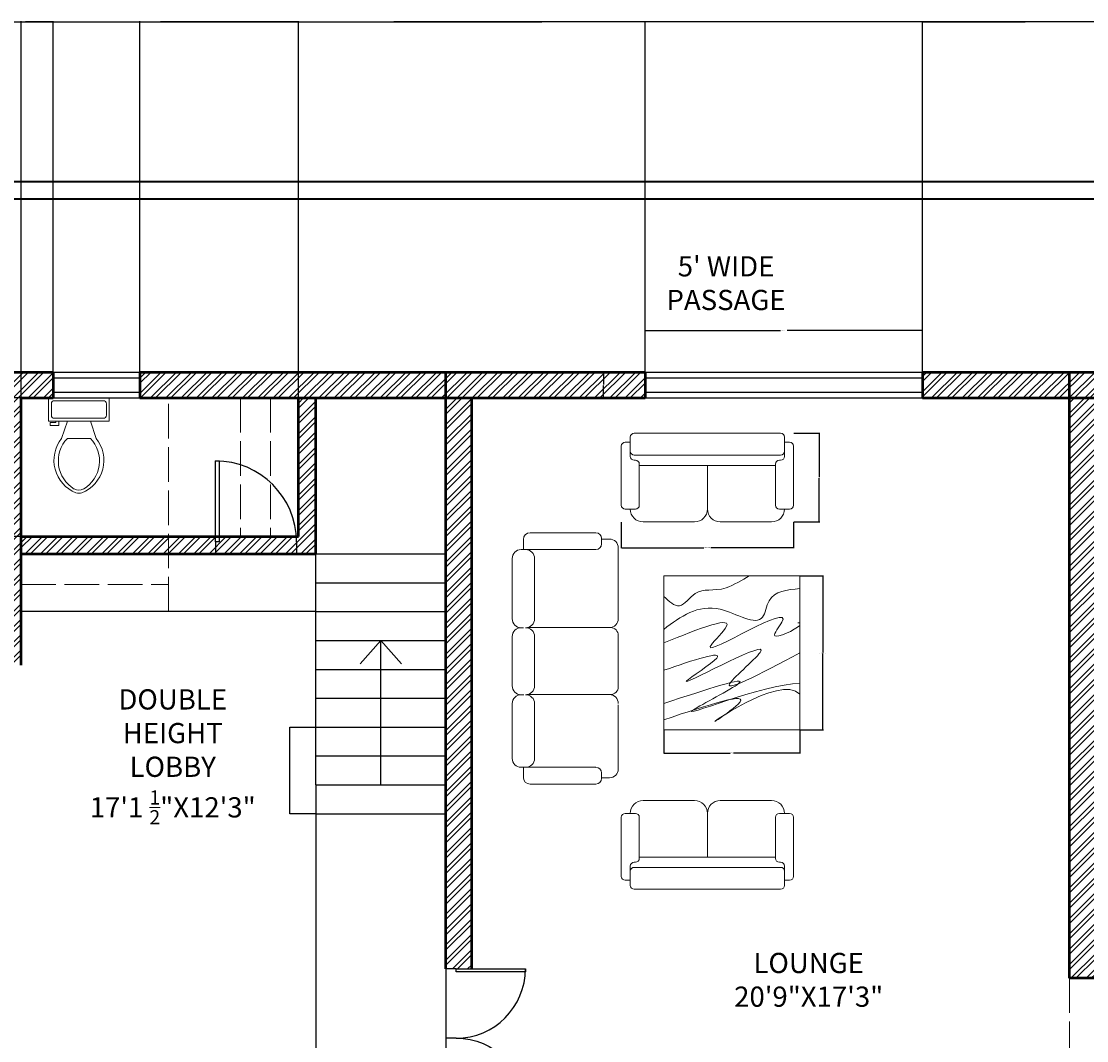
# Model space of a CAD drawing. Units: inches. Extents: x -249 to 953, y -127 to 590.
# Tile 3 of 4: x 171 to 540, y 237 to 590. Entities that reach past the tile are written whole.
import ezdxf

# ---------------------------------------------------------------- set-up
doc = ezdxf.new("R2010")
doc.units = ezdxf.units.IN
doc.header["$MEASUREMENT"] = 0
doc.linetypes.add('ACAD_ISO02W100', pattern=[15, 12, -3])
for name, color, linetype, lineweight in [('A-ANNO-DIMS', 2, 'Continuous', 18), ('A-AREA-IDEN', 2, 'Continuous', 18), ('A-FLOR-STRS', 4, 'Continuous', 25), ('A-FLOR-STRS-OVHD', 4, 'ACAD_ISO02W100', 18), ('A-FURN', 42, 'Continuous', 18), ('A-GLAZ', 5, 'Continuous', 25), ('A-WALL', 7, 'Continuous', 50), ('A-WALL-OVHD', 7, 'ACAD_ISO02W100', 18), ('A-WALL-PATT', 8, 'Continuous', 13), ('C-PROP', 7, 'Continuous', 35), ('DOOR', 22, 'Continuous', 25), ('L-ANNO-TEXT', 2, 'Continuous', 18), ('WASHROOM', 2, 'Continuous', 18)]:
    doc.layers.add(name, color=color, linetype=linetype, lineweight=lineweight)
doc.styles.get("Standard").update_dxf_attribs({"font": 'arial.ttf'})
doc.dimstyles.get("Standard").update_dxf_attribs({"dimtxt": 0.18, "dimasz": 0.18, "dimexe": 0.18, "dimexo": 0.0625, "dimgap": 0.09, "dimtad": 0, "dimtih": 1, "dimtoh": 1, "dimdec": 4, "dimzin": 0, "dimdsep": 46, "dimtxsty": 'Standard', "dimcen": 0.09, "dimadec": 0, "dimazin": 0, "dimtfac": 1, "dimtdec": 4, "dimtofl": 0, "dimtmove": 0, "dimatfit": 3, "dimfxl": 1, "dimtolj": 1, "dimtzin": 0, "dimarcsym": 0})

# ---------------------------------------------------------------- blocks, each defined once
blk = doc.blocks.new('*U2')
for p, q in [((0, 0), (0, -6)), ((40, 0), (40, -6))]:
    blk.add_line(p, q)
blk.add_lwpolyline([(0, 0), (0, 40), (1.75, 40), (1.75, 0)], close=True)
blk.add_arc((0, 0), 40, 0, 90)
blk = doc.blocks.new('A$C0876780F')
for p, q in [((0.15, 0.87), (0.15, 0.8444)), ((0.15, 0.87), (0.15, 0.85)), ((0.72, 0.95), (0.23, 0.95)), ((0.8, 0.85), (0.8, 0.87)), ((0.8, 0.87), (0.8, 0.85)), ((0.8, 0.87), (0.8, 0.8444)), ((1.32, 0.95), (0.88, 0.95)), ((1.4, 0.85), (1.4, 0.87)), ((1.4, 0.85), (1.4, 0.87)), ((1.48, 0.95), (2.02, 0.95)), ((2.1, 0.87), (2.1, 0.85)), ((2.1, 0.87), (2.1, 0.8444)), ((0, 0.79), (0, 0.21)), ((0.15, 0.85), (0.06, 0.85)), ((0.15, 0.21), (0.15, 0.85)), ((0.8011, 0.8204), (0.8011, 0.08)), ((1.4014, 0.08), (1.4014, 0.803)), ((2.1, 0.21), (2.1, 0.85)), ((2.1, 0.85), (2.19, 0.85)), ((2.25, 0.79), (2.25, 0.21)), ((0.72, 0.75), (0.23, 0.75)), ((1.32, 0.75), (0.88, 0.75)), ((1.48, 0.75), (2.02, 0.75)), ((0, 0.21), (0, 0.2)), ((0.15, 0.2), (0.15, 0.25)), ((2.1, 0.2), (2.1, 0.25)), ((2.25, 0.21), (2.25, 0.2)), ((0.05, 0.15), (0.1, 0.15)), ((0.056, 0.15), (0.056, 0.08)), ((2.2, 0.15), (2.15, 0.15)), ((2.194, 0.15), (2.194, 0.08)), ((0.136, 0), (0.7093, 0)), ((0.8011, 0.07), (0.8011, 0.08)), ((0.8711, 0), (1.3314, 0)), ((1.4014, 0.07), (1.4014, 0.08)), ((2.114, 0), (1.48, 0))]:
    blk.add_line(p, q)
for centre, radius, start, end in [((0.23, 0.87), 0.08, 90, 180), ((0.72, 0.87), 0.08, 0, 90), ((0.88, 0.87), 0.08, 90, 180), ((1.32, 0.87), 0.08, 0, 90), ((1.48, 0.87), 0.08, 90, 180), ((2.02, 0.87), 0.08, 0, 90), ((0.06, 0.79), 0.06, 90, 180), ((0.23, 0.83), 0.08, 180, 270), ((0.23, 0.83), 0.08, 180, 270), ((0.72, 0.83), 0.08, 270, 0), ((0.88, 0.83), 0.08, 180, 270), ((0.88, 0.83), 0.08, 180, 270), ((1.32, 0.83), 0.08, 270, 0), ((1.48, 0.83), 0.08, 180, 270), ((2.02, 0.83), 0.08, 270, 0), ((2.02, 0.83), 0.08, 270, 0), ((2.19, 0.79), 0.06, 0, 90), ((0.05, 0.2), 0.05, 180, 270), ((0.1, 0.2), 0.05, 270, 0), ((0.09, 0.21), 0.06, 350.53768, 0), ((2.16, 0.21), 0.06, 180, 189.46232), ((2.15, 0.2), 0.05, 180, 270), ((2.2, 0.2), 0.05, 270, 0), ((0.136, 0.08), 0.08, 180, 270), ((0.7211, 0.08), 0.08, 270, 0), ((0.8711, 0.07), 0.07, 180, 270), ((1.3314, 0.07), 0.07, 270, 0), ((1.4814, 0.08), 0.08, 180, 270), ((2.114, 0.08), 0.08, 270, 0)]:
    blk.add_arc(centre, radius, start, end)
blk = doc.blocks.new('A$C02A636C4')
for p, q in [((1.2026, 0.6692), (0.097, 0.6692)), ((0, 0.5722), (0, 0.1261)), ((0.0679, 0.6013), (0.0291, 0.6013)), ((0.0679, 0.6401), (0.0679, 0.6013)), ((0.0679, 0.5334), (0.0679, 0.6013)), ((1.2317, 0.6401), (1.2317, 0.6013)), ((1.2317, 0.6013), (1.2705, 0.6013)), ((1.2317, 0.5334), (1.2317, 0.6013)), ((1.2996, 0.5722), (1.2996, 0.1261)), ((0.0679, 0.4946), (0.0679, 0.5431)), ((1.2026, 0.5043), (0.097, 0.5043)), ((1.2317, 0.4946), (1.2317, 0.5431)), ((0.1067, 0.4655), (0.097, 0.4655)), ((0.1358, 0.1261), (0.1358, 0.4364)), ((1.1638, 0.4267), (0.1358, 0.4267)), ((0.6498, 0.097), (0.6498, 0.4267)), ((1.1638, 0.1261), (1.1638, 0.4364)), ((1.1929, 0.4655), (1.2026, 0.4655)), ((0.0291, 0.097), (0.1067, 0.097)), ((1.2705, 0.097), (1.1929, 0.097)), ((0.1649, 0), (0.5528, 0)), ((0.7468, 0), (1.1347, 0))]:
    blk.add_line(p, q)
for centre, radius, start, end in [((0.097, 0.6401), 0.0291, 90, 180), ((1.2026, 0.6401), 0.0291, 0, 90), ((0.0291, 0.5722), 0.0291, 90, 180), ((1.2705, 0.5722), 0.0291, 0, 90), ((0.097, 0.5334), 0.0291, 180, 270), ((0.097, 0.4946), 0.0291, 180, 270), ((1.2026, 0.5334), 0.0291, 270, 0), ((1.2026, 0.4946), 0.0291, 270, 0), ((0.1067, 0.4364), 0.0291, 0, 90), ((1.1929, 0.4364), 0.0291, 90, 180), ((0.0291, 0.1261), 0.0291, 180, 270), ((0.1649, 0.097), 0.097, 180, 270), ((0.1067, 0.1261), 0.0291, 270, 0), ((0.5528, 0.097), 0.097, 270, 0), ((0.7468, 0.097), 0.097, 180, 270), ((1.1347, 0.097), 0.097, 270, 0), ((1.1929, 0.1261), 0.0291, 180, 270), ((1.2705, 0.1261), 0.0291, 270, 0)]:
    blk.add_arc(centre, radius, start, end)
blk = doc.blocks.new('*U11')
for p, q in [((241.3, -152.4), (241.3, -50.8)), ((-254, -215.9), (-203.2, -215.9)), ((-254, -241.3), (-254, -215.9)), ((-177.8, -241.3), (-254, -241.3)), ((-203.2, -215.9), (-203.2, -203.2)), ((-177.8, -203.2), (-177.8, -241.3)), ((-101.6, -203.2), (-152.4, -355.6)), ((101.6, -203.2), (152.4, -355.6)), ((101.6, -355.6), (-101.6, -355.6))]:
    blk.add_line(p, q)
blk.add_lwpolyline([(266.7, -203.2), (266.7, 0), (-266.7, 0), (-266.7, -203.2)], close=True)
for points in [[(-241.3, -50.8), (-241.3, -152.4)], [(215.9, -25.4), (-215.9, -25.4)], [(-215.9, -177.8), (215.9, -177.8)]]:
    blk.add_lwpolyline(points)
for centre, radius, start, end in [((-219.1, -47.6), 22.5, 81.8699, 188.1301), ((219.1, -47.6), 22.5, 351.8699, 98.1301), ((-219.1, -155.6), 22.5, 171.8699, 278.1301), ((219.1, -155.6), 22.5, 261.8699, 8.1301), ((89.4, -548.1), 309.1, 141.46911, 247.97143), ((106.7, -554.2), 287.8, 136.36773, 238.94682), ((-89.4, -548.1), 309.1, 292.02843, 38.53071), ((-106.7, -554.2), 287.8, 301.05301, 43.63209), ((0, -708.1), 101.6, 245.73182, 294.26817), ((0, -736.6), 101.6, 254.86053, 285.13947)]:
    blk.add_arc(centre, radius, start, end)
blk = doc.blocks.new('TABLE-COFFEE-PATTERNED')
blk.add_lwpolyline([(0, 53.34), (47.12, 53.34), (47.12, 0), (0, 0)], close=True)
for points, knots in [([(0, 46.27), (1.84, 44.53), (5.7, 40.88), (11.7, 50.21), (19.06, 46.91), (27.14, 52), (29.62, 53.34)], [0, 0, 0, 0, 6.282368, 13.190835, 24.063381, 30.451568, 30.451568, 30.451568, 30.451568]), ([(0, 34.85), (5.86, 39.26), (15.94, 46.83), (34.57, 34.01), (35.96, 47.88), (42.72, 48.56), (47.12, 49)], [0, 0, 0, 0, 20.758426, 35.677626, 41.810907, 53.27251, 53.27251, 53.27251, 53.27251]), ([(0, 30.13), (12.39, 35.14), (29.39, 42), (5.27, 19.44), (51.08, 48.6), (34.79, 29.62), (45.43, 34.67), (47.12, 36.21)], [0, 0, 0, 0, 21.871026, 29.981696, 56.235396, 61.567804, 69.030503, 69.030503, 69.030503, 69.030503]), ([(0, 20.7), (10.31, 24.19), (27.82, 30.11), (-7.6, 7.42), (48.95, 38.75), (11.44, 7.85), (33.32, 19.39), (47.12, 26.67)], [0, 0, 0, 0, 18.796744, 31.916986, 59.888518, 75.000199, 100.823224, 100.823224, 100.823224, 100.823224]), ([(0, 3.52), (15.31, 8.65), (36.14, 15.62), (5.39, -5.65), (40.11, 19.54), (47.12, 12.46)], [0, 0, 0, 0, 26.265752, 35.743864, 66.169502, 66.169502, 66.169502, 66.169502]), ([(0, 9.16), (14.7, 14.03), (39.32, 22.19), (-9.44, -2.68), (34.4, 16.08), (47.12, 16.13)], [0, 0, 0, 0, 26.807232, 44.891452, 82.87087, 82.87087, 82.87087, 82.87087])]:
    blk.add_open_spline(points, degree=3, knots=knots)
blk.add_open_spline([(47.12, 37.08), (46.93, 37.1), (46.67, 37.09), (46.41, 37.08)], degree=3)
blk = doc.blocks.new('WIN-30IN')
for p, q in [((0, 9), (30, 9)), ((0, 7), (30, 7)), ((0, 2), (30, 2)), ((0, 0), (30, 0))]:
    blk.add_line(p, q)
blk = doc.blocks.new('WIN-96IN')
for p, q in [((0, 9), (96, 9)), ((0, 7), (96, 7)), ((0, 2), (96, 2)), ((0, 0), (96, 0))]:
    blk.add_line(p, q)
blk = doc.blocks.new('*D29')
at = {"layer": 'A-ANNO-DIMS', "color": 0, "lineweight": -2, "transparency": 16777216}
for p, q in [((379.03, 416.95), (379.03, 407.89)), ((438.67, 416.95), (438.67, 407.89)), ((379.21, 408.07), (407.63, 408.07)), ((438.49, 408.07), (410.07, 408.07))]:
    blk.add_line(p, q, dxfattribs=at)
at = {"layer": 'A-ANNO-DIMS', "color": 0, "transparency": 16777216}
for points in [[(379.21, 408.1), (379.21, 408.04), (379.03, 408.07)], [(438.49, 408.1), (438.49, 408.04), (438.67, 408.07)]]:
    blk.add_solid(points, dxfattribs=at)
at = {"layer": 'Defpoints', "color": 0, "transparency": 16777216}
for p in [(379.03, 417.02), (438.67, 417.02), (438.67, 408.07)]:
    blk.add_point(p, dxfattribs=at)
at = {"layer": 'A-ANNO-DIMS', "color": 0, "transparency": 16777216, "insert": (408.85, 408.07), "char_height": 0.18, "attachment_point": 5}
blk.add_mtext('\\A1;LOVESEAT 60 TYP.', dxfattribs=at)
blk = doc.blocks.new('*D30')
at = {"layer": 'A-ANNO-DIMS', "color": 0, "lineweight": -2, "transparency": 16777216}
for p, q in [((438.73, 447.72), (447.79, 447.72)), ((447.61, 447.54), (447.61, 432.55)), ((447.61, 417.2), (447.61, 432.19)), ((438.73, 417.02), (447.79, 417.02))]:
    blk.add_line(p, q, dxfattribs=at)
at = {"layer": 'A-ANNO-DIMS', "color": 0, "transparency": 16777216}
for points in [[(447.58, 447.54), (447.64, 447.54), (447.61, 447.72)], [(447.58, 417.2), (447.64, 417.2), (447.61, 417.02)]]:
    blk.add_solid(points, dxfattribs=at)
at = {"layer": 'Defpoints', "color": 0, "transparency": 16777216}
for p in [(438.67, 447.72), (447.61, 447.72), (438.67, 417.02)]:
    blk.add_point(p, dxfattribs=at)
at = {"layer": 'A-ANNO-DIMS', "color": 0, "transparency": 16777216, "insert": (447.61, 432.37), "char_height": 0.18, "attachment_point": 5}
blk.add_mtext('\\A1;31 TYP.', dxfattribs=at)
blk = doc.blocks.new('*D37')
at = {"layer": 'A-ANNO-DIMS', "color": 0, "lineweight": -2, "transparency": 16777216}
for p, q in [((440.93, 398.27), (449.04, 398.27)), ((448.86, 398.09), (448.86, 371.78)), ((448.86, 345.11), (448.86, 371.42)), ((440.93, 344.93), (449.04, 344.93))]:
    blk.add_line(p, q, dxfattribs=at)
at = {"layer": 'A-ANNO-DIMS', "color": 0, "transparency": 16777216}
for points in [[(448.83, 398.09), (448.89, 398.09), (448.86, 398.27)], [(448.83, 345.11), (448.89, 345.11), (448.86, 344.93)]]:
    blk.add_solid(points, dxfattribs=at)
at = {"layer": 'Defpoints', "color": 0, "transparency": 16777216}
for p in [(440.86, 398.27), (448.86, 398.27), (440.86, 344.93)]:
    blk.add_point(p, dxfattribs=at)
at = {"layer": 'A-ANNO-DIMS', "color": 0, "transparency": 16777216, "insert": (448.86, 371.6), "char_height": 0.18, "attachment_point": 5}
blk.add_mtext('\\A1;COFFEE TABLE 53 TYP.', dxfattribs=at)
blk = doc.blocks.new('*D38')
at = {"layer": 'A-ANNO-DIMS', "color": 0, "lineweight": -2, "transparency": 16777216}
for p, q in [((393.74, 344.87), (393.74, 336.75)), ((440.86, 344.87), (440.86, 336.75)), ((393.92, 336.93), (416.77, 336.93)), ((440.68, 336.93), (417.84, 336.93))]:
    blk.add_line(p, q, dxfattribs=at)
at = {"layer": 'A-ANNO-DIMS', "color": 0, "transparency": 16777216}
for points in [[(393.92, 336.96), (393.92, 336.9), (393.74, 336.93)], [(440.68, 336.96), (440.68, 336.9), (440.86, 336.93)]]:
    blk.add_solid(points, dxfattribs=at)
at = {"layer": 'Defpoints', "color": 0, "transparency": 16777216}
for p in [(393.74, 344.93), (440.86, 344.93), (440.86, 336.93)]:
    blk.add_point(p, dxfattribs=at)
at = {"layer": 'A-ANNO-DIMS', "color": 0, "transparency": 16777216, "insert": (417.3, 336.93), "char_height": 0.18, "attachment_point": 5}
blk.add_mtext('\\A1;47 TYP.', dxfattribs=at)
blk = doc.blocks.new('*D43')
at = {"layer": 'A-ANNO-DIMS', "color": 0, "lineweight": -2, "transparency": 16777216}
for p, q in [((387.31, 468.99), (387.31, 483.51)), ((483.31, 468.99), (483.31, 483.51)), ((387.49, 483.33), (434.19, 483.33)), ((483.13, 483.33), (436.42, 483.33))]:
    blk.add_line(p, q, dxfattribs=at)
at = {"layer": 'A-ANNO-DIMS', "color": 0, "transparency": 16777216}
for points in [[(387.49, 483.36), (387.49, 483.3), (387.31, 483.33)], [(483.13, 483.36), (483.13, 483.3), (483.31, 483.33)]]:
    blk.add_solid(points, dxfattribs=at)
at = {"layer": 'Defpoints', "color": 0, "transparency": 16777216}
for p in [(483.31, 483.33), (387.31, 468.93), (483.31, 468.93)]:
    blk.add_point(p, dxfattribs=at)
at = {"layer": 'A-ANNO-DIMS', "color": 0, "transparency": 16777216, "insert": (435.31, 483.33), "char_height": 0.18, "attachment_point": 5}
blk.add_mtext('\\A1;WINDOW 96 TYP.', dxfattribs=at)
blk = doc.blocks.new('*D44')
at = {"layer": 'A-ANNO-DIMS', "color": 0, "lineweight": -2, "transparency": 16777216}
for p, q in [((387.24, 468.93), (372.73, 468.93)), ((372.91, 468.75), (372.91, 464.61)), ((372.91, 460.11), (372.91, 464.25)), ((387.24, 459.93), (372.73, 459.93))]:
    blk.add_line(p, q, dxfattribs=at)
at = {"layer": 'A-ANNO-DIMS', "color": 0, "transparency": 16777216}
for points in [[(372.88, 468.75), (372.94, 468.75), (372.91, 468.93)], [(372.88, 460.11), (372.94, 460.11), (372.91, 459.93)]]:
    blk.add_solid(points, dxfattribs=at)
at = {"layer": 'Defpoints', "color": 0, "transparency": 16777216}
for p in [(372.91, 468.93), (387.31, 468.93), (387.31, 459.93)]:
    blk.add_point(p, dxfattribs=at)
at = {"layer": 'A-ANNO-DIMS', "color": 0, "transparency": 16777216, "insert": (372.91, 464.43), "char_height": 0.18, "attachment_point": 5}
blk.add_mtext('\\A1;9 TYP.', dxfattribs=at)
blk = doc.blocks.new('*D51')
at = {"layer": 'A-ANNO-DIMS', "color": 0, "lineweight": -2, "transparency": 16777216}
for p, q in [((-193.28, 534.99), (-193.28, 590.41)), ((897.22, 534.99), (897.22, 590.41)), ((-193.1, 590.23), (351.51, 590.23)), ((897.04, 590.23), (352.42, 590.23))]:
    blk.add_line(p, q, dxfattribs=at)
at = {"layer": 'A-ANNO-DIMS', "color": 0, "transparency": 16777216}
for points in [[(-193.1, 590.26), (-193.1, 590.2), (-193.28, 590.23)], [(897.04, 590.26), (897.04, 590.2), (897.22, 590.23)]]:
    blk.add_solid(points, dxfattribs=at)
at = {"layer": 'Defpoints', "color": 0, "transparency": 16777216}
for p in [(897.22, 590.23), (-193.28, 534.93), (897.22, 534.93)]:
    blk.add_point(p, dxfattribs=at)
at = {"layer": 'A-ANNO-DIMS', "color": 0, "transparency": 16777216, "insert": (351.97, 590.23), "char_height": 0.18, "attachment_point": 5}
blk.add_mtext('\\A1;1090.5', dxfattribs=at)
blk = doc.blocks.new('*D59')
at = {"layer": 'A-ANNO-DIMS', "color": 0, "lineweight": -2, "transparency": 16777216}
for p, q in [((273.22, 325.87), (273.22, -126.55)), ((318.22, 325.87), (318.22, -126.55)), ((273.4, -126.37), (295.49, -126.37)), ((318.04, -126.37), (295.94, -126.37))]:
    blk.add_line(p, q, dxfattribs=at)
at = {"layer": 'A-ANNO-DIMS', "color": 0, "transparency": 16777216}
for points in [[(273.4, -126.34), (273.4, -126.4), (273.22, -126.37)], [(318.04, -126.34), (318.04, -126.4), (318.22, -126.37)]]:
    blk.add_solid(points, dxfattribs=at)
at = {"layer": 'Defpoints', "color": 0, "transparency": 16777216}
for p in [(273.22, 325.93), (318.22, 325.93), (318.22, -126.37)]:
    blk.add_point(p, dxfattribs=at)
at = {"layer": 'A-ANNO-DIMS', "color": 0, "transparency": 16777216, "insert": (295.72, -126.37), "char_height": 0.18, "attachment_point": 5}
blk.add_mtext('\\A1;45', dxfattribs=at)
blk = doc.blocks.new('*D60')
at = {"layer": 'A-ANNO-DIMS', "color": 0, "lineweight": -2, "transparency": 16777216}
for p, q in [((171.22, 411.99), (171.22, 590.41)), ((267.22, 411.99), (267.22, 590.41)), ((171.4, 590.23), (219, 590.23)), ((267.04, 590.23), (219.43, 590.23))]:
    blk.add_line(p, q, dxfattribs=at)
at = {"layer": 'A-ANNO-DIMS', "color": 0, "transparency": 16777216}
for points in [[(171.4, 590.26), (171.4, 590.2), (171.22, 590.23)], [(267.04, 590.26), (267.04, 590.2), (267.22, 590.23)]]:
    blk.add_solid(points, dxfattribs=at)
at = {"layer": 'Defpoints', "color": 0, "transparency": 16777216}
for p in [(267.22, 590.23), (171.22, 411.93), (267.22, 411.93)]:
    blk.add_point(p, dxfattribs=at)
at = {"layer": 'A-ANNO-DIMS', "color": 0, "transparency": 16777216, "insert": (219.22, 590.23), "char_height": 0.18, "attachment_point": 5}
blk.add_mtext('\\A1;96', dxfattribs=at)
blk = doc.blocks.new('*D61')
at = {"layer": 'A-ANNO-DIMS', "color": 0, "lineweight": -2, "transparency": 16777216}
for p, q in [((171.15, 459.93), (-248.76, 459.93)), ((-248.58, 459.75), (-248.58, 436.11)), ((-248.58, 412.11), (-248.58, 435.75)), ((171.15, 411.93), (-248.76, 411.93))]:
    blk.add_line(p, q, dxfattribs=at)
at = {"layer": 'A-ANNO-DIMS', "color": 0, "transparency": 16777216}
for points in [[(-248.61, 459.75), (-248.55, 459.75), (-248.58, 459.93)], [(-248.61, 412.11), (-248.55, 412.11), (-248.58, 411.93)]]:
    blk.add_solid(points, dxfattribs=at)
at = {"layer": 'Defpoints', "color": 0, "transparency": 16777216}
for p in [(-248.58, 459.93), (171.22, 459.93), (171.22, 411.93)]:
    blk.add_point(p, dxfattribs=at)
at = {"layer": 'A-ANNO-DIMS', "color": 0, "transparency": 16777216, "insert": (-248.58, 435.93), "char_height": 0.18, "attachment_point": 5}
blk.add_mtext('\\A1;48', dxfattribs=at)
blk = doc.blocks.new('*D62')
at = {"layer": 'A-ANNO-DIMS', "color": 0, "lineweight": -2, "transparency": 16777216}
for p, q in [((162.22, 468.99), (162.22, 590.41)), ((182.27, 468.99), (182.27, 590.41)), ((162.4, 590.23), (171.78, 590.23)), ((182.09, 590.23), (172.71, 590.23))]:
    blk.add_line(p, q, dxfattribs=at)
at = {"layer": 'A-ANNO-DIMS', "color": 0, "transparency": 16777216}
for points in [[(162.4, 590.26), (162.4, 590.2), (162.22, 590.23)], [(182.09, 590.26), (182.09, 590.2), (182.27, 590.23)]]:
    blk.add_solid(points, dxfattribs=at)
at = {"layer": 'Defpoints', "color": 0, "transparency": 16777216}
for p in [(182.27, 590.23), (162.22, 468.93), (182.27, 468.93)]:
    blk.add_point(p, dxfattribs=at)
at = {"layer": 'A-ANNO-DIMS', "color": 0, "transparency": 16777216, "insert": (172.24, 590.23), "char_height": 0.18, "attachment_point": 5}
blk.add_mtext('\\A1;20.058', dxfattribs=at)
blk = doc.blocks.new('*D63')
at = {"layer": 'A-ANNO-DIMS', "color": 0, "lineweight": -2, "transparency": 16777216}
for p, q in [((212.27, 468.99), (212.27, 590.41)), ((387.31, 468.99), (387.31, 590.41)), ((212.45, 590.23), (299.33, 590.23)), ((387.13, 590.23), (300.24, 590.23))]:
    blk.add_line(p, q, dxfattribs=at)
at = {"layer": 'A-ANNO-DIMS', "color": 0, "transparency": 16777216}
for points in [[(212.45, 590.26), (212.45, 590.2), (212.27, 590.23)], [(387.13, 590.26), (387.13, 590.2), (387.31, 590.23)]]:
    blk.add_solid(points, dxfattribs=at)
at = {"layer": 'Defpoints', "color": 0, "transparency": 16777216}
for p in [(387.31, 590.23), (212.27, 468.93), (387.31, 468.93)]:
    blk.add_point(p, dxfattribs=at)
at = {"layer": 'A-ANNO-DIMS', "color": 0, "transparency": 16777216, "insert": (299.79, 590.23), "char_height": 0.18, "attachment_point": 5}
blk.add_mtext('\\A1;175.03', dxfattribs=at)
blk = doc.blocks.new('*D64')
at = {"layer": 'A-ANNO-DIMS', "color": 0, "lineweight": -2, "transparency": 16777216}
for p, q in [((483.31, 468.99), (483.31, 590.41)), ((555.26, 468.99), (555.26, 590.41)), ((483.49, 590.23), (518.89, 590.23)), ((555.08, 590.23), (519.68, 590.23))]:
    blk.add_line(p, q, dxfattribs=at)
at = {"layer": 'A-ANNO-DIMS', "color": 0, "transparency": 16777216}
for points in [[(483.49, 590.26), (483.49, 590.2), (483.31, 590.23)], [(555.08, 590.26), (555.08, 590.2), (555.26, 590.23)]]:
    blk.add_solid(points, dxfattribs=at)
at = {"layer": 'Defpoints', "color": 0, "transparency": 16777216}
for p in [(555.26, 590.23), (483.31, 468.93), (555.26, 468.93)]:
    blk.add_point(p, dxfattribs=at)
at = {"layer": 'A-ANNO-DIMS', "color": 0, "transparency": 16777216, "insert": (519.28, 590.23), "char_height": 0.18, "attachment_point": 5}
blk.add_mtext('\\A1;71.96', dxfattribs=at)

msp = doc.modelspace()

# ---------------------------------------------------------------- hatches: boundary and pattern name
at = {"layer": 'A-WALL-PATT'}
h = msp.add_hatch(dxfattribs=at)
h.set_pattern_fill('ANSI32', color=256, scale=10)
h.paths.add_polyline_path([(387.3054, 468.9306), (318.2157, 468.9306), (318.2157, 459.9306), (387.3054, 459.9306)])
h.paths.add_polyline_path([(327.2157, 459.9306), (318.2157, 459.9306), (318.2157, 262.174), (321.8157, 262.174), (327.2157, 262.174)])
h.paths.add_polyline_path([(318.2157, 468.9306), (212.2733, 468.9306), (212.2733, 459.9306), (318.2157, 459.9306)])
h.paths.add_polyline_path([(182.2733, 468.9306), (162.2157, 468.9306), (162.2157, 367.3439), (171.2157, 367.3439), (171.2157, 459.9306), (182.2733, 459.9306)])
h = msp.add_hatch(dxfattribs=at)
h.set_pattern_fill('ANSI32', color=256, scale=10)
h.paths.add_polyline_path([(678.2396, 468.9306), (585.2636, 468.9306), (585.2636, 459.9306), (678.2396, 459.9306)])
h.paths.add_polyline_path([(555.2636, 468.9306), (534.2157, 468.9306), (534.2157, 459.9306), (555.2636, 459.9306)])
h.paths.add_polyline_path([(534.2157, 468.9306), (483.3054, 468.9306), (483.3054, 459.9306), (534.2157, 459.9306)])
h.paths.add_polyline_path([(543.2157, 459.9306), (534.2157, 459.9306), (534.2157, 258.9306), (543.2157, 258.9306)])
h = msp.add_hatch(dxfattribs=at)
h.set_pattern_fill('ANSI32', color=256, scale=10)
h.paths.add_polyline_path([(222.2157, 411.9306), (171.2157, 411.9306), (171.2157, 405.9306), (222.2157, 405.9306)])
h.paths.add_polyline_path([(238.5143, 410.1306), (238.5143, 411.9306), (222.2157, 411.9306), (222.2157, 405.9306), (238.5143, 405.9306)])
h.paths.add_polyline_path([(266.5143, 410.1306, 0.01608391), (266.4563, 411.9306), (239.7393, 411.9306), (239.7393, 410.1306), (238.5143, 410.1306), (238.5143, 405.9306), (266.5143, 405.9306)])
h.paths.add_polyline_path([(273.2157, 459.9306), (267.2157, 459.9306), (267.2157, 411.9306), (266.4563, 411.9306, -0.01608391), (266.5143, 410.1306), (266.5143, 405.9306), (273.2157, 405.9306)])

# ---------------------------------------------------------------- linework, layer by layer
at = {"layer": 'A-FLOR-STRS'}
for p, q in [((273.2157, 405.9306), (318.2157, 405.9306)), ((273.2157, 325.9306), (273.2157, 405.9306)), ((273.2157, 395.9306), (318.2157, 395.9306)), ((273.2157, 385.9306), (171.2157, 385.9306)), ((273.2157, 385.9306), (318.2157, 385.9306)), ((273.2157, 375.9306), (318.2157, 375.9306)), ((295.7157, 375.9306), (288.5782, 367.8092)), ((295.7157, 325.9306), (295.7157, 375.9306)), ((295.7157, 375.9306), (302.8532, 367.8092)), ((273.2157, 365.9306), (318.2157, 365.9306)), ((273.2157, 355.9306), (318.2157, 355.9306)), ((264.2157, 315.9306), (264.2157, 345.9306)), ((264.2157, 345.9306), (273.2157, 345.9306)), ((273.2157, 345.9306), (318.2157, 345.9306)), ((273.2157, 335.9306), (318.2157, 335.9306)), ((273.2157, 325.9306), (318.2157, 325.9306)), ((273.2157, 315.9306), (264.2157, 315.9306)), ((273.2157, 315.9306), (318.2157, 315.9306))]:
    msp.add_line(p, q, dxfattribs=at)
at = {"layer": 'A-FLOR-STRS-OVHD'}
for p, q in [((222.2157, 385.9306), (222.2157, 459.9306)), ((247.1126, 459.9306), (247.1126, 411.9306)), ((257.5136, 459.9306), (257.5136, 411.9306)), ((171.2157, 395.2753), (222.2157, 395.2753))]:
    msp.add_line(p, q, dxfattribs=at)
at = {"layer": 'A-WALL'}
for p, q in [((162.2157, 468.9306), (182.2733, 468.9306)), ((182.2733, 468.9306), (182.2733, 459.9306)), ((212.2733, 468.9306), (212.2733, 459.9306)), ((212.2733, 468.9306), (387.3054, 468.9306)), ((318.2157, 262.174), (318.2157, 468.9306)), ((387.3054, 468.9306), (387.3054, 459.9306)), ((483.3054, 468.9306), (483.3054, 459.9306)), ((483.3054, 468.9306), (555.2636, 468.9306)), ((534.2157, 258.9306), (534.2157, 468.9306)), ((171.2157, 459.9306), (182.2733, 459.9306)), ((171.2157, 367.3439), (171.2157, 459.9306)), ((212.2733, 459.9306), (387.3054, 459.9306)), ((267.2157, 411.9306), (267.2157, 459.9306)), ((273.2157, 405.9306), (273.2157, 459.9306)), ((327.2157, 262.174), (327.2157, 459.9306)), ((483.3054, 459.9306), (555.2636, 459.9306)), ((171.2157, 411.9306), (267.2157, 411.9306)), ((171.2157, 405.9306), (273.2157, 405.9306)), ((543.2157, 258.9306), (534.2157, 258.9306))]:
    msp.add_line(p, q, dxfattribs=at)
at = {"layer": 'A-WALL-OVHD'}
msp.add_line((534.2157, 258.9306), (534.2157, 210.9306), dxfattribs=at)
at = {"layer": 'C-PROP'}
for p, q in [((-193.2843, 534.9306), (897.2157, 534.9306)), ((-187.2843, 528.9306), (891.2157, 528.9306))]:
    msp.add_line(p, q, dxfattribs=at)

# ---------------------------------------------------------------- block references
at = {"layer": 'A-FURN', "xscale": 45.88752760856259, "yscale": 45.88752760856259, "zscale": 45.88752760856259}
msp.add_blockref('A$C02A636C4', (379.0331, 417.0151), dxfattribs=at)
at = {"layer": 'A-FURN'}
for name, p, xscale, yscale, zscale, rotation in [('A$C0876780F', (377.9864, 326.1983), 38.68315051238548, 38.68315051238548, 38.68315051238548, 90), ('A$C02A636C4', (379.0331, 320.4844), -45.88752760856259, 45.88752760856259, 45.88752760856259, 180)]:
    msp.add_blockref(name, p, dxfattribs=dict(at, xscale=xscale, yscale=yscale, zscale=zscale, rotation=rotation))
msp.add_blockref('TABLE-COFFEE-PATTERNED', (393.7438, 344.9324), dxfattribs=at)
at = {"layer": 'A-GLAZ'}
for name, p in [('WIN-30IN', (182.273, 459.931)), ('WIN-96IN', (387.305, 459.931))]:
    msp.add_blockref(name, p, dxfattribs=at)
at = {"layer": 'DOOR', "xscale": 0.7000000000000001, "yscale": 0.7000000000000001, "zscale": 0.7000000000000001}
msp.add_blockref('*U2', (238.5143, 410.1306), dxfattribs=at)
at = {"layer": 'DOOR', "yscale": 0.6, "zscale": 0.6, "rotation": 270}
for p, xscale in [((321.8157, 262.174), 0.6), ((321.8157, 214.174), -0.6)]:
    msp.add_blockref('*U2', p, dxfattribs=dict(at, xscale=xscale))
at = {"layer": 'WASHROOM', "xscale": 0.0393700787401575, "yscale": 0.0393700787401575, "zscale": 0.0393700787401575}
msp.add_blockref('*U11', (191.1681, 459.9306), dxfattribs=at)

# ---------------------------------------------------------------- texts
at = {"layer": 'A-AREA-IDEN', "char_height": 7, "attachment_point": 1}
for s, insert in [('\\A1;\\pxqc;DOUBLE\\PHEIGHT\\PLOBBY\\P17\'1 {\\H0.7x;\\S1/2;}"X12\'3"', (183.8564, 359.0225)), ('\\A1;\\pxqc;LOUNGE\\P20\'9"X17\'3"', (404.1247, 267.7241))]:
    msp.add_mtext_dynamic_manual_height_columns(s, width=79.609867, gutter_width=1, heights=[0], dxfattribs=dict(at, insert=insert))
at = {"layer": 'L-ANNO-TEXT', "insert": (375.4991, 509.052), "char_height": 7, "attachment_point": 1}
msp.add_mtext_dynamic_manual_height_columns("\\A1;\\pxqc;5' WIDE\\PPASSAGE", width=79.609867, gutter_width=1, heights=[0], dxfattribs=at)

# ---------------------------------------------------------------- dimensions: what is measured, and where the dimension line sits
at = {"layer": 'A-ANNO-DIMS'}
for base, p1, p2, override, picture, middle in [((897.2157, 590.2306), (-193.2843, 534.9306), (897.2157, 534.9306), {"dimdec": 1, "dimlfac": 1, "dimrnd": 0, "dimzin": 0, "dimdsep": 46, "dimlunit": 2}, '*D51', (351.9657, 590.2306)), ((182.2733, 590.2306), (162.2157, 468.9306), (182.2733, 468.9306), {"dimdec": 3, "dimlfac": 1, "dimrnd": 0, "dimzin": 0, "dimdsep": 46, "dimlunit": 2}, '*D62', (172.2445, 590.2306)), ((267.2157, 590.2306), (171.2157, 411.9306), (267.2157, 411.9306), {"dimdec": 0, "dimlfac": 1, "dimrnd": 0, "dimzin": 0, "dimdsep": 46, "dimlunit": 2}, '*D60', (219.2157, 590.2306)), ((387.3054, 590.2306), (212.2733, 468.9306), (387.3054, 468.9306), {"dimdec": 2, "dimlfac": 1, "dimrnd": 0, "dimzin": 0, "dimdsep": 46, "dimlunit": 2}, '*D63', (299.7893, 590.2306)), ((555.2636, 590.2306), (483.3054, 468.9306), (555.2636, 468.9306), {"dimdec": 2, "dimlfac": 1, "dimrnd": 0, "dimzin": 0, "dimdsep": 46, "dimlunit": 2}, '*D64', (519.2845, 590.2306)), ((318.2157, -126.3694), (273.2157, 325.9306), (318.2157, 325.9306), {"dimdec": 0, "dimlfac": 1, "dimrnd": 0, "dimzin": 0, "dimdsep": 46, "dimlunit": 2}, '*D59', (295.7157, -126.3694))]:
    dim = msp.add_linear_dim(base=base, p1=p1, p2=p2, dimstyle='Standard', override=override, dxfattribs=at)
    dim.commit()
    dim.dimension.update_dxf_attribs({"geometry": picture, "text_midpoint": middle})
for base, p1, p2, text, picture, middle in [((483.3054, 483.3306), (387.3054, 468.9306), (483.3054, 468.9306), 'WINDOW <> TYP.', '*D43', (435.3054, 483.3306)), ((438.6695, 408.0697), (379.0331, 417.0151), (438.6695, 417.0151), 'LOVESEAT <> TYP.', '*D29', (408.8513, 408.0697)), ((440.8642, 336.9318), (393.744, 344.9323), (440.8642, 344.9323), '<> TYP.', '*D38', (417.3041, 336.9318))]:
    dim = msp.add_linear_dim(base=base, p1=p1, p2=p2, text=text, dimstyle='Standard', override={"dimdec": 0, "dimlfac": 1, "dimrnd": 0, "dimzin": 0, "dimdsep": 46, "dimlunit": 2}, dxfattribs=at)
    dim.commit()
    dim.dimension.update_dxf_attribs({"geometry": picture, "text_midpoint": middle})
for base, p1, p2, text, picture, middle in [((372.9054, 468.9306), (387.3054, 459.9306), (387.3054, 468.9306), '<> TYP.', '*D44', (372.9054, 464.4306)), ((447.6149, 447.7234), (438.6695, 417.0151), (438.6695, 447.7234), '<> TYP.', '*D30', (447.6149, 432.3693)), ((448.8648, 398.2695), (440.8642, 344.9323), (440.8642, 398.2695), 'COFFEE TABLE <> TYP.', '*D37', (448.8648, 371.6009))]:
    dim = msp.add_linear_dim(base=base, p1=p1, p2=p2, angle=90, text=text, dimstyle='Standard', override={"dimdec": 0, "dimlfac": 1, "dimrnd": 0, "dimzin": 0, "dimdsep": 46, "dimlunit": 2}, dxfattribs=at)
    dim.commit()
    dim.dimension.update_dxf_attribs({"geometry": picture, "text_midpoint": middle})
dim = msp.add_linear_dim(base=(-248.5843, 459.9306), p1=(171.2157, 411.9306), p2=(171.2157, 459.9306), angle=90, dimstyle='Standard', override={"dimdec": 0, "dimlfac": 1, "dimrnd": 0, "dimzin": 0, "dimdsep": 46, "dimlunit": 2}, dxfattribs=at)
dim.commit()
dim.dimension.update_dxf_attribs({"geometry": '*D61', "text_midpoint": (-248.5843, 435.9306)})

doc.saveas('drawing.dxf')
